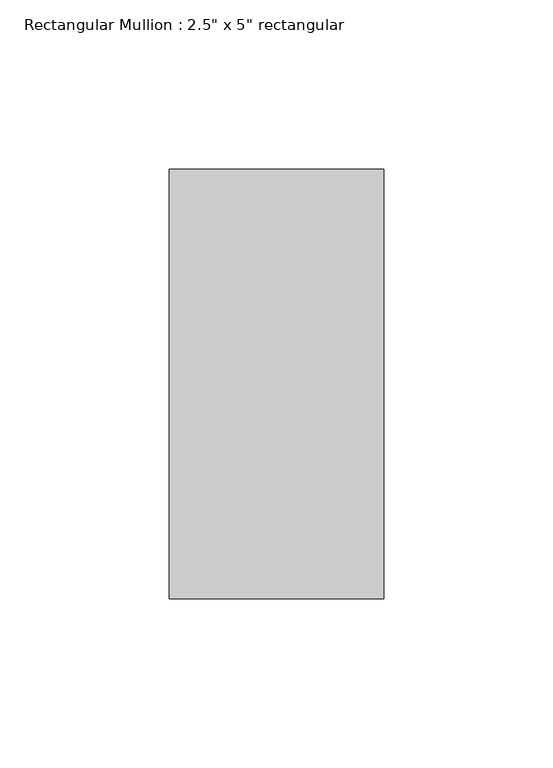
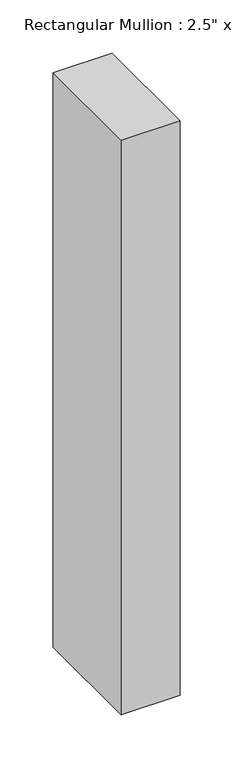
"""IFC4 building model written with IfcOpenShell, lengths in millimetres: member geometry."""

from ifc_helpers import new_model, si_unit, frame, origin, place, context, project, spatial, polyline, outline, extrude, source, transform, mapped, element, save


def member_297e028d(model_context):
    return source(origin(), model_context, "Body", "SweptSolid", [
        extrude(outline(polyline([(0.0, 63.5), (0.0, -63.5), (-63.5, -63.5), (-63.5, 63.5), (0.0, 63.5)])), frame((0.0, 0.0, -656.1666667), z_axis=(0.0, 0.0, 1.0), x_axis=(1.0, 0.0, 0.0)), (0.0, 0.0, 1.0), 656.1666667),
    ])


if __name__ == "__main__":
    model = new_model("IFC4")
    model_context = context("Model", 3, world=origin())
    ifc_project = project(units=[si_unit("LENGTHUNIT", "METRE", prefix="MILLI")], contexts=[model_context])
    site = spatial("IfcSite", under=ifc_project)
    building = spatial("IfcBuilding", under=site)
    placement = place(None, origin())
    member_shape = member_297e028d(model_context)
    element("IfcMember", 1, ObjectType="Rectangular Mullion : 2.5\" x 5\" rectangular", at=placement, inside=building, context=model_context, shape_type="MappedRepresentation", body=[
        mapped(member_shape, transform((0.0, 0.0, 0.0), x_axis=(1.0, 0.0, 0.0), y_axis=(0.0, 1.0, 0.0), z_axis=(0.0, 0.0, 1.0))),
    ])
    save(model, "model.ifc")

# Revit data of these elements
# Type "Rectangular Mullion : 2.5\" x 5\" rectangular"
#   built-in parameter 1007304 = 0.416667 (stored number, unit not read)
#   built-in parameter 1007301 = 0.104167 (stored number, unit not read)
#   built-in parameter 1007300 = 0.104167 (stored number, unit not read)
# Element 1 (IfcMember, "Rectangular Mullion : 2.5\" x 5\" rectangular")
#   Materials on its faces: "Aluminum"
# Materials
#   "Aluminum": class "Metal", colour RGB 247 247 247, transparency 0, Description = "Aluminum 6061", Cost = 0
